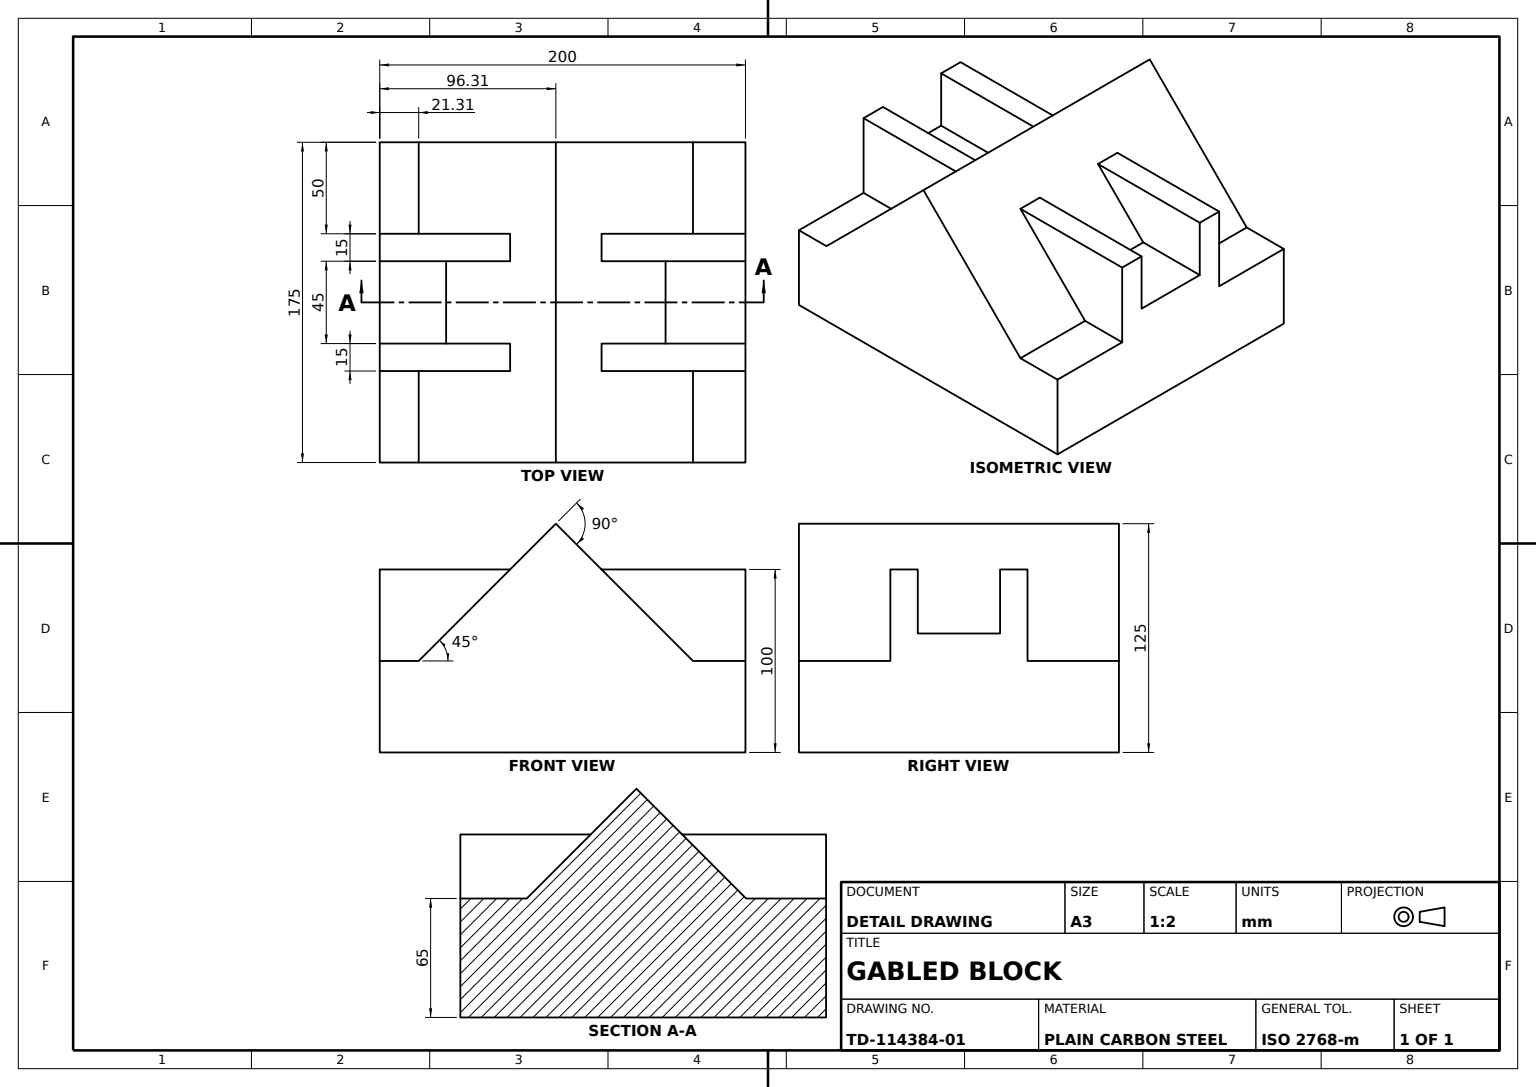
from build123d import *

# Parameters (mm, degrees)
BASE_WEDGE_BLOCK_DEPTH = 87.5
TWIN_START             = -200
TWIN_SLOTS_15MM_DEPTH  = 200


with BuildPart() as part:
    # Base Profile Sketch → Base Wedge Block (new, symmetric)
    with BuildSketch(Plane.XY):
        Polygon((-96.311034199, 0), (103.688965801, 0), (103.688965801, 50), (75, 50), (0, 125), (-75, 50), (-96.311034199, 50), align=None)
    extrude(amount=BASE_WEDGE_BLOCK_DEPTH, both=True)

    # Slot Profile Sketch → Twin Slots 15mm (add)
    with BuildSketch(Plane(origin=(103.688965801, 0, 0), x_dir=(0, 0, -1), z_dir=(1, 0, 0)).offset(TWIN_START)):
        Polygon((-87.5, 0), (-87.5, 50), (-37.5, 50), (-37.5, 100), (-22.5, 100), (-22.5, 65), (22.5, 65), (22.5, 100), (37.5, 100), (37.5, 50), (87.5, 50), (87.5, 0), align=None)
    extrude(amount=TWIN_SLOTS_15MM_DEPTH)


solid = part.part
